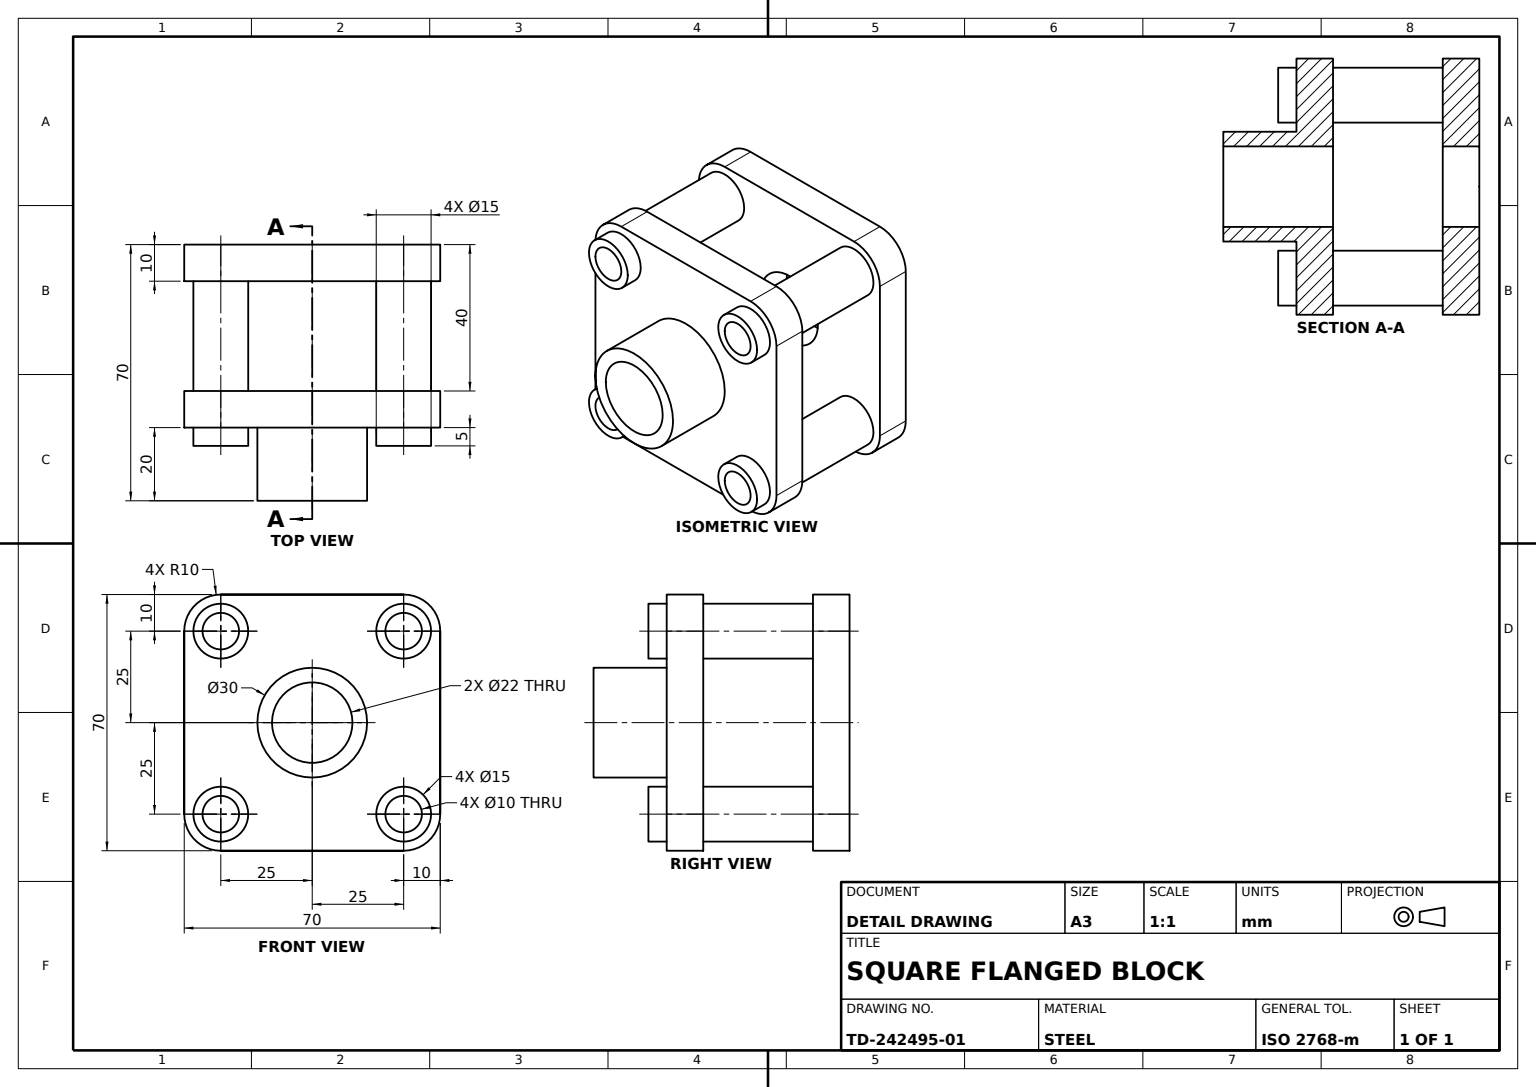
SolidWorks part; units mm, degrees
material "Plain Carbon Steel"
ref_plane "Front Plane" through (0, 0, 0) normal (0, 0, 1) x (1, 0, 0)
ref_plane "Top Plane" through (0, 0, 0) normal (0, 1, 0) x (1, 0, 0)
ref_plane "Right Plane" through (0, 0, 0) normal (1, 0, 0) x (0, 0, -1)
sketch "Base Plate Sketch" plane through (0, 0, 0) normal (0, 0, 1) x (1, 0, 0)
  line L0 (0, 0) -> (70, 0)
  line L1 (70, 0) -> (70, 70)
  line L2 (70, 70) -> (0, 70)
  line L3 (0, 70) -> (0, 0)
  dimension "D1" = 70
  dimension "D2" = 70
extrude "Base Plate" add sketch "Base Plate Sketch" along normal blind 10
sketch "Corner Posts Sketch" plane through (0, 0, 10) normal (0, 0, 1) x (1, 0, 0)
  line L0 (0, 0) -> (10, 0) construction
  line L1 (0, 0) -> (70, 0) construction
  line L2 (10, 0) -> (10, 10) construction
  line L3 (70, 0) -> (60, 0) construction
  line L4 (60, 0) -> (60, 10) construction
  line L5 (70, 70) -> (60, 70) construction
  line L6 (70, 70) -> (0, 70) construction
  line L7 (60, 70) -> (60, 60) construction
  line L8 (0, 70) -> (10, 70) construction
  line L9 (10, 70) -> (10, 60) construction
  line L10 (0, 70) -> (0, 0) construction
  circle A0 centre (10, 10) radius 7.5
  circle A1 centre (60, 10) radius 7.5
  circle A2 centre (60, 60) radius 7.5
  circle A3 centre (10, 60) radius 7.5
  dimension "D1" = 15
  dimension "D2" = 15
  dimension "D3" = 15
  dimension "D4" = 15
  dimension "D5" = 10
extrude "Corner Posts 4x" add sketch "Corner Posts Sketch" along normal blind 30
ref_plane "Top Plate Plane" through (0, 0, 40) normal (0, 0, 1) x (1, 0, 0)
sketch "Top Plate Sketch" plane through (0, 0, 40) normal (0, 0, 1) x (1, 0, 0)
  line L0 (0, 70) -> (70, 70)
  line L1 (70, 70) -> (70, 0)
  line L2 (70, 0) -> (0, 0)
  line L3 (0, 0) -> (0, 70)
extrude "Top Plate" add sketch "Top Plate Sketch" along normal blind 10
sketch "Post Bosses Sketch" plane through (0, 0, 50) normal (0, 0, 1) x (1, 0, 0)
  line L0 (0, 70) -> (10, 70) construction
  line L1 (70, 70) -> (0, 70) construction
  line L2 (10, 70) -> (10, 60) construction
  line L3 (70, 70) -> (60, 70) construction
  line L4 (60, 70) -> (60, 60) construction
  line L5 (0, 0) -> (10, 0) construction
  line L6 (0, 0) -> (70, 0) construction
  line L7 (10, 0) -> (10, 10) construction
  line L8 (0, 70) -> (0, 0) construction
  circle A0 centre (10, 60) radius 5
  circle A1 centre (10, 60) radius 7.5
  circle A2 centre (60, 60) radius 5
  circle A3 centre (60, 60) radius 7.5
  circle A4 centre (10, 10) radius 5
  circle A5 centre (10, 10) radius 7.5
  circle A6 centre (60, 10) radius 5
  circle A7 centre (60, 10) radius 7.5
  dimension "D1" = 15
  dimension "D2" = 10
  dimension "D3" = 15
  dimension "D4" = 10
  dimension "D5" = 10
  dimension "D6" = 15
  dimension "D7" = 15
  dimension "D8" = 10
  dimension "D9" = 10
extrude "Post Bosses 4x" add sketch "Post Bosses Sketch" along normal blind 5
sketch "Centre Boss Sketch" plane through (0, 0, 50) normal (0, 0, 1) x (1, 0, 0)
  circle A0 centre (35, 35) radius 11
  circle A1 centre (35, 35) radius 15
  circle A2 centre (10, 60) radius 7.5 construction
  dimension "D1" = 30
  dimension "D2" = 22
  dimension "D3" = 25
  dimension "D4" = 25
extrude "Centre Boss Ø30" add sketch "Centre Boss Sketch" along normal blind 20
sketch "Centre Bore Sketch" plane through (0, 0, 50) normal (0, 0, 1) x (1, 0, 0)
  circle A0 centre (35, 35) radius 11
  dimension "D1" = 22
extrude "Centre Bore Cut" cut sketch "Centre Bore Sketch" against normal through all
sketch "Post Holes Sketch" plane through (0, 0, 50) normal (0, 0, 1) x (1, 0, 0)
  circle A0 centre (60, 60) radius 5
  circle A1 centre (10, 60) radius 5
  circle A2 centre (60, 10) radius 5
  circle A3 centre (10, 10) radius 5
  dimension "D1" = 10
extrude "Post Holes 4x" cut sketch "Post Holes Sketch" against normal through all
fillet "Top Plate Corner Fillets R10" radius 10 4 edges at (70, 70, 45) (0, 70, 45) (0, 0, 45) (70, 0, 45)
fillet "Base Plate Corner Fillets R10" radius 10 4 edges at (70, 70, 5) (70, 0, 5) (0, 0, 5) (0, 70, 5)
